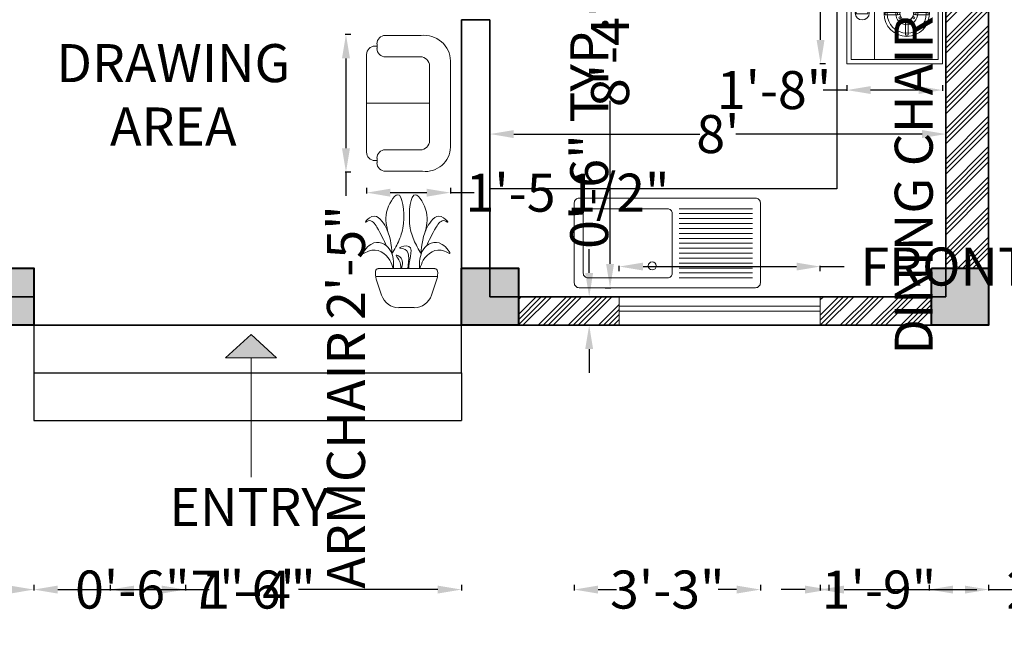
# Model space of a CAD drawing. Units: inches. Extents: x -52 to 493, y -432 to 100.
# Tile 2 of 5: x 163 to 370, y -432 to -300. Entities that reach past the tile are written whole.
import ezdxf

# ---------------------------------------------------------------- set-up
doc = ezdxf.new("R2010")
doc.units = ezdxf.units.IN
doc.header["$MEASUREMENT"] = 0
for name, color, linetype, lineweight in [('A-ANNO-DIMS', 2, 'Continuous', 18), ('A-ANNO-SYMB', 7, 'Continuous', 18), ('A-ANNO-TEXT', 7, 'Continuous', 25), ('A-AREA-IDEN', 7, 'Continuous', 25), ('A-COLS', 7, 'Continuous', 40), ('A-EQPM', 8, 'Continuous', 18), ('A-FLOR-CASE', 8, 'Continuous', 25), ('A-FLOR-FIXT', 9, 'Continuous', 18), ('A-FLOR-FIXT-PATT', 9, 'Continuous', 13), ('A-FLOR-STRS', 7, 'Continuous', 25), ('A-FURN', 8, 'Continuous', 18), ('A-GLAZ', 4, 'Continuous', 18), ('A-WALL', 7, 'Continuous', 35), ('A-WALL-PATT', 8, 'Continuous', 13)]:
    doc.layers.add(name, color=color, linetype=linetype, lineweight=lineweight)
doc.styles.get("Standard").update_dxf_attribs({"font": 'arial.ttf'})
doc.dimstyles.get("Standard").update_dxf_attribs({"dimtxt": 8, "dimasz": 5, "dimexe": 0.18, "dimexo": 0.0625, "dimgap": 0.09, "dimtad": 0, "dimdec": 0, "dimzin": 0, "dimdsep": 46, "dimlunit": 3, "dimtxsty": 'Standard', "dimcen": 0.09, "dimadec": 0, "dimazin": 0, "dimtfac": 1, "dimtdec": 0, "dimtofl": 0, "dimtmove": 0, "dimatfit": 3, "dimfxl": 1, "dimfxlon": 1, "dimtolj": 1, "dimtzin": 0, "dimarcsym": 0})

# ---------------------------------------------------------------- blocks, each defined once
blk = doc.blocks.new('A$C6D011943')
for p, q in [((1.448, 1.089), (0.332, 1.089)), ((1.364, 0.818), (0.398, 0.818)), ((0.881, 0.818), (0.881, 0)), ((0, 0.709), (0, 0.247)), ((0.278, 0.697), (0.278, 0.244)), ((1.485, 0.244), (1.485, 0.697)), ((1.762, 0.247), (1.762, 0.727)), ((0.109, 0.136), (0.169, 0.136)), ((0.139, 0.109), (0.139, 0.136)), ((1.593, 0.136), (1.654, 0.136)), ((1.648, 0.136), (1.623, 0.136)), ((1.623, 0.109), (1.623, 0.136)), ((1.515, 0), (0.247, 0))]:
    blk.add_line(p, q)
for centre, radius, start, end in [((0.339, 0.748), 0.342, 91.2564, 186.501), ((1.441, 0.766), 0.324, 353.159, 88.6697), ((0.398, 0.697), 0.121, 90, 180), ((1.364, 0.697), 0.121, 0, 90), ((0.109, 0.244), 0.109, 180, 270), ((0.169, 0.244), 0.109, 270, 0), ((1.593, 0.244), 0.109, 180, 270), ((1.654, 0.244), 0.109, 270, 0), ((0.247, 0.109), 0.109, 180, 270), ((1.515, 0.109), 0.109, 270, 0)]:
    blk.add_arc(centre, radius, start, end)
blk = doc.blocks.new('A$C06E242FC')
for p, q in [((0, 455.6), (0.5, 456.1)), ((0, 455.6), (0, 0.5)), ((838.9, 456.1), (0.5, 456.1)), ((20, 435.6), (20.5, 436.1)), ((20, 435.6), (20, 20.5)), ((818.9, 436.1), (20.5, 436.1)), ((819.4, 435.6), (818.9, 436.1)), ((819.4, 20.5), (819.4, 435.6)), ((838.9, 456.1), (839.4, 455.6)), ((839.4, 0.5), (839.4, 455.6)), ((237.3, 411.5), (237.3, 356.2)), ((248.9, 411.5), (237.3, 411.5)), ((248.9, 356.2), (248.9, 411.5)), ((599.3, 411.5), (610.9, 411.5)), ((599.3, 411.5), (599.3, 356.2)), ((610.9, 356.2), (610.9, 411.5)), ((237.3, 356.2), (248.9, 356.2)), ((599.3, 356.2), (610.9, 356.2)), ((20, 324.4), (819.4, 324.4)), ((232.7, 272.7), (232.7, 214)), ((244.9, 272.7), (232.7, 272.7)), ((244.9, 214), (244.9, 272.7)), ((588.1, 272.7), (588.1, 214)), ((600.3, 272.7), (588.1, 272.7)), ((600.3, 214), (600.3, 272.7)), ((232.7, 214), (244.9, 214)), ((588.1, 214), (600.3, 214)), ((136.3, 176), (136.3, 163.8)), ((194.9, 176), (136.3, 176)), ((136.3, 163.8), (194.9, 163.8)), ((194.9, 163.8), (194.9, 176)), ((282.9, 176.3), (282.9, 164.1)), ((341.6, 176.3), (282.9, 176.3)), ((282.9, 164.1), (341.6, 164.1)), ((341.6, 164.1), (341.6, 176.3)), ((550.3, 176), (491.7, 176)), ((491.7, 176), (491.7, 163.8)), ((491.7, 163.8), (550.3, 163.8)), ((550.3, 163.8), (550.3, 176)), ((638.3, 176.3), (638.3, 164.1)), ((697, 176.3), (638.3, 176.3)), ((638.3, 164.1), (697, 164.1)), ((697, 164.1), (697, 176.3)), ((245.2, 126.1), (233, 126.1)), ((233, 126.1), (233, 67.4)), ((245.2, 67.4), (245.2, 126.1)), ((600.6, 126.1), (588.3, 126.1)), ((588.3, 126.1), (588.3, 67.4)), ((600.6, 67.4), (600.6, 126.1)), ((233, 67.4), (245.2, 67.4)), ((588.3, 67.4), (600.6, 67.4)), ((0, 0.5), (0.5, 0)), ((20, 20.5), (20.5, 20)), ((20.5, 20), (818.9, 20)), ((818.9, 20), (819.4, 20.5)), ((838.9, 0), (839.4, 0.5)), ((0.5, 0), (838.9, 0))]:
    blk.add_line(p, q)
for centre, radius in [((242, 382.9), 33.3), ((604.1, 382.9), 33.3), ((238.9, 170.1), 108.3), ((238.9, 170.1), 93.3), ((594.3, 170.1), 108.3), ((594.3, 170.1), 93.3), ((238.9, 170.1), 52.6), ((205.3, 189.5), 4.84), ((238.9, 170.1), 32.6), ((219.5, 203.7), 4.84), ((238.9, 208.9), 4.84), ((258.4, 203.7), 4.84), ((272.6, 189.5), 4.84), ((594.3, 170.1), 52.6), ((560.7, 189.5), 4.84), ((594.3, 170.1), 32.6), ((574.9, 203.7), 4.84), ((594.3, 208.9), 4.84), ((613.7, 203.7), 4.84), ((628, 189.5), 4.84), ((200.1, 170.1), 4.84), ((205.3, 150.6), 4.84), ((219.5, 136.4), 4.84), ((258.4, 136.4), 4.84), ((272.6, 150.6), 4.84), ((277.8, 170.1), 4.84), ((555.5, 170.1), 4.84), ((560.7, 150.6), 4.84), ((574.9, 136.4), 4.84), ((613.7, 136.4), 4.84), ((628, 150.6), 4.84), ((633.2, 170.1), 4.84), ((238.9, 131.2), 4.84), ((594.3, 131.2), 4.84)]:
    blk.add_circle(centre, radius)
blk = doc.blocks.new('*D19')
at = {"layer": 'A-ANNO-DIMS', "color": 0, "lineweight": -2, "transparency": 16777216}
for p, q in [((285.94, -256.62), (287.12, -256.62)), ((286.94, -261.62), (286.94, -295.94)), ((286.94, -351.72), (286.94, -317.4)), ((285.94, -356.72), (287.12, -356.72))]:
    blk.add_line(p, q, dxfattribs=at)
at = {"layer": 'A-ANNO-DIMS', "color": 0, "transparency": 16777216}
for points in [[(286.11, -261.62), (287.78, -261.62), (286.94, -256.62)], [(286.11, -351.72), (287.78, -351.72), (286.94, -356.72)]]:
    blk.add_solid(points, dxfattribs=at)
at = {"layer": 'Defpoints', "color": 0, "transparency": 16777216}
for p in [(283.02, -256.62), (280.41, -356.72), (286.94, -356.72)]:
    blk.add_point(p, dxfattribs=at)
at = {"layer": 'A-ANNO-DIMS', "color": 0, "transparency": 16777216, "insert": (286.94, -306.67), "char_height": 8, "attachment_point": 5, "rotation": 90}
blk.add_mtext('\\A1;8\'-4"', dxfattribs=at)
blk = doc.blocks.new('*D20')
at = {"layer": 'A-ANNO-DIMS', "color": 0, "lineweight": -2, "transparency": 16777216}
for p, q in [((261.65, -323.39), (261.65, -324.57)), ((266.65, -324.39), (305.87, -324.39)), ((352.65, -324.39), (313.42, -324.39)), ((357.65, -323.39), (357.65, -324.57))]:
    blk.add_line(p, q, dxfattribs=at)
at = {"layer": 'A-ANNO-DIMS', "color": 0, "transparency": 16777216}
for points in [[(266.65, -323.56), (266.65, -325.23), (261.65, -324.39)], [(352.65, -323.56), (352.65, -325.23), (357.65, -324.39)]]:
    blk.add_solid(points, dxfattribs=at)
at = {"layer": 'Defpoints', "color": 0, "transparency": 16777216}
for p in [(261.65, -318.52), (357.65, -318.52), (357.65, -324.39)]:
    blk.add_point(p, dxfattribs=at)
at = {"layer": 'A-ANNO-DIMS', "color": 0, "transparency": 16777216, "insert": (309.65, -324.39), "char_height": 8, "attachment_point": 5}
blk.add_mtext("\\A1;8'", dxfattribs=at)
blk = doc.blocks.new('COL-12X12')
h = blk.add_hatch(color=256)
h.dxf.hatch_style = 1
h.paths.add_polyline_path([(12, 12), (0, 12), (0, 0), (12, 0)])
blk.add_lwpolyline([(0, 12), (12, 12), (12, 0), (0, 0)], close=True)
blk = doc.blocks.new('WIN-FRONT-42')
for p, q in [((0, 6), (0, 0)), ((42.31, 6), (42.31, 0)), ((42.31, 4), (0, 4)), ((42.31, 3), (0, 3))]:
    blk.add_line(p, q)
blk = doc.blocks.new('*D36')
at = {"layer": 'A-ANNO-DIMS', "color": 0, "lineweight": -2, "transparency": 16777216}
for p, q in [((288.89, -353.27), (288.89, -352.09)), ((293.89, -352.27), (326.2, -352.27)), ((331.2, -353.27), (331.2, -352.09)), ((331.2, -352.27), (336.2, -352.27))]:
    blk.add_line(p, q, dxfattribs=at)
at = {"layer": 'A-ANNO-DIMS', "color": 0, "transparency": 16777216}
for points in [[(293.89, -351.44), (293.89, -353.1), (288.89, -352.27)], [(326.2, -351.44), (326.2, -353.1), (331.2, -352.27)]]:
    blk.add_solid(points, dxfattribs=at)
at = {"layer": 'Defpoints', "color": 0, "transparency": 16777216}
for p in [(331.2, -352.27), (288.89, -358.62), (331.2, -358.62)]:
    blk.add_point(p, dxfattribs=at)
at = {"layer": 'A-ANNO-DIMS', "color": 0, "transparency": 16777216, "insert": (416.63, -352.27), "char_height": 8, "attachment_point": 5}
blk.add_mtext('\\A1;FRONT WINDOW 3\'-6 1/2" TYP.', dxfattribs=at)
blk = doc.blocks.new('*D37')
at = {"layer": 'A-ANNO-DIMS', "color": 0, "lineweight": -2, "transparency": 16777216}
for p, q in [((282.55, -353.62), (282.55, -348.62)), ((283.55, -358.62), (282.37, -358.62)), ((283.55, -364.62), (282.37, -364.62)), ((282.55, -369.62), (282.55, -374.62))]:
    blk.add_line(p, q, dxfattribs=at)
at = {"layer": 'A-ANNO-DIMS', "color": 0, "transparency": 16777216}
for points in [[(281.71, -353.62), (283.38, -353.62), (282.55, -358.62)], [(281.71, -369.62), (283.38, -369.62), (282.55, -364.62)]]:
    blk.add_solid(points, dxfattribs=at)
at = {"layer": 'Defpoints', "color": 0, "transparency": 16777216}
for p in [(282.55, -358.62), (288.89, -358.62), (288.89, -364.62)]:
    blk.add_point(p, dxfattribs=at)
at = {"layer": 'A-ANNO-DIMS', "color": 0, "transparency": 16777216, "insert": (282.55, -324.14), "char_height": 8, "attachment_point": 5, "rotation": 90}
blk.add_mtext('\\A1;0\'-6" TYP.', dxfattribs=at)
blk = doc.blocks.new('*D44')
at = {"layer": 'A-ANNO-DIMS', "color": 0, "lineweight": -2, "transparency": 16777216}
for p, q in [((349.88, -208.05), (351.06, -208.05)), ((350.88, -213.05), (350.88, -216.46)), ((349.88, -221.46), (351.06, -221.46)), ((350.88, -221.46), (350.88, -226.46))]:
    blk.add_line(p, q, dxfattribs=at)
at = {"layer": 'A-ANNO-DIMS', "color": 0, "transparency": 16777216}
for points in [[(350.04, -213.05), (351.71, -213.05), (350.88, -208.05)], [(350.04, -216.46), (351.71, -216.46), (350.88, -221.46)]]:
    blk.add_solid(points, dxfattribs=at)
at = {"layer": 'Defpoints', "color": 0, "transparency": 16777216}
for p in [(348.87, -208.05), (348.87, -221.46), (350.88, -221.46)]:
    blk.add_point(p, dxfattribs=at)
at = {"layer": 'A-ANNO-DIMS', "color": 0, "transparency": 16777216, "insert": (350.88, -300.1), "char_height": 8, "attachment_point": 5, "rotation": 90}
blk.add_mtext('\\A1;DINING CHAIR 1\'-1 1/2" TYP.', dxfattribs=at)
blk = doc.blocks.new('*D52')
at = {"layer": 'A-ANNO-DIMS', "color": 0, "lineweight": -2, "transparency": 16777216}
for p, q in [((232.34, -303.47), (231.16, -303.47)), ((231.34, -308.47), (231.34, -327.39)), ((232.34, -332.39), (231.16, -332.39)), ((231.34, -332.39), (231.34, -337.39))]:
    blk.add_line(p, q, dxfattribs=at)
at = {"layer": 'A-ANNO-DIMS', "color": 0, "transparency": 16777216}
for points in [[(230.51, -308.47), (232.18, -308.47), (231.34, -303.47)], [(230.51, -327.39), (232.18, -327.39), (231.34, -332.39)]]:
    blk.add_solid(points, dxfattribs=at)
at = {"layer": 'Defpoints', "color": 0, "transparency": 16777216}
for p in [(235.68, -303.47), (231.34, -332.39), (235.68, -332.39)]:
    blk.add_point(p, dxfattribs=at)
at = {"layer": 'A-ANNO-DIMS', "color": 0, "transparency": 16777216, "insert": (231.34, -379.7), "char_height": 8, "attachment_point": 5, "rotation": 90}
blk.add_mtext('\\A1;ARMCHAIR 2\'-5"', dxfattribs=at)
blk = doc.blocks.new('*D53')
at = {"layer": 'A-ANNO-DIMS', "color": 0, "lineweight": -2, "transparency": 16777216}
for p, q in [((235.68, -335.72), (235.68, -336.9)), ((253.34, -335.72), (253.34, -336.9)), ((240.68, -336.72), (248.34, -336.72)), ((253.34, -336.72), (258.34, -336.72))]:
    blk.add_line(p, q, dxfattribs=at)
at = {"layer": 'A-ANNO-DIMS', "color": 0, "transparency": 16777216}
for points in [[(240.68, -335.89), (240.68, -337.56), (235.68, -336.72)], [(248.34, -335.89), (248.34, -337.56), (253.34, -336.72)]]:
    blk.add_solid(points, dxfattribs=at)
at = {"layer": 'Defpoints', "color": 0, "transparency": 16777216}
for p in [(235.68, -332.39), (253.34, -332.39), (253.34, -336.72)]:
    blk.add_point(p, dxfattribs=at)
at = {"layer": 'A-ANNO-DIMS', "color": 0, "transparency": 16777216, "insert": (278, -336.72), "char_height": 8, "attachment_point": 5}
blk.add_mtext('\\A1;1\'-5 1/2"', dxfattribs=at)
blk = doc.blocks.new('*D54')
at = {"layer": 'A-ANNO-DIMS', "color": 0, "lineweight": -2, "transparency": 16777216}
for p, q in [((331.27, -272.61), (331.27, -267.61)), ((332.27, -272.61), (331.09, -272.61)), ((331.27, -304.59), (331.27, -277.61)), ((332.27, -309.59), (331.09, -309.59))]:
    blk.add_line(p, q, dxfattribs=at)
at = {"layer": 'A-ANNO-DIMS', "color": 0, "transparency": 16777216}
for points in [[(330.43, -277.61), (332.1, -277.61), (331.27, -272.61)], [(330.43, -304.59), (332.1, -304.59), (331.27, -309.59)]]:
    blk.add_solid(points, dxfattribs=at)
at = {"layer": 'Defpoints', "color": 0, "transparency": 16777216}
for p in [(331.27, -272.61), (336.81, -272.61), (336.81, -309.59)]:
    blk.add_point(p, dxfattribs=at)
at = {"layer": 'A-ANNO-DIMS', "color": 0, "transparency": 16777216, "insert": (331.27, -227.44), "char_height": 8, "attachment_point": 5, "rotation": 90}
blk.add_mtext('\\A1;COOKTOP 3\'-1"', dxfattribs=at)
blk = doc.blocks.new('*D55')
at = {"layer": 'A-ANNO-DIMS', "color": 0, "lineweight": -2, "transparency": 16777216}
for p, q in [((336.81, -314.14), (336.81, -315.32)), ((356.91, -314.14), (356.91, -315.32)), ((336.81, -315.14), (331.81, -315.14)), ((351.91, -315.14), (341.81, -315.14))]:
    blk.add_line(p, q, dxfattribs=at)
at = {"layer": 'A-ANNO-DIMS', "color": 0, "transparency": 16777216}
for points in [[(341.81, -314.31), (341.81, -315.97), (336.81, -315.14)], [(351.91, -314.31), (351.91, -315.97), (356.91, -315.14)]]:
    blk.add_solid(points, dxfattribs=at)
at = {"layer": 'Defpoints', "color": 0, "transparency": 16777216}
for p in [(336.81, -309.59), (356.91, -309.59), (336.81, -315.14)]:
    blk.add_point(p, dxfattribs=at)
at = {"layer": 'A-ANNO-DIMS', "color": 0, "transparency": 16777216, "insert": (321.47, -315.14), "char_height": 8, "attachment_point": 5}
blk.add_mtext('\\A1;1\'-8"', dxfattribs=at)
blk = doc.blocks.new('*D64')
at = {"layer": 'A-ANNO-DIMS', "color": 0, "lineweight": -2, "transparency": 16777216}
for p, q in [((101.4, -419.22), (101.4, -420.4)), ((106.4, -420.22), (113.48, -420.22)), ((160.65, -420.22), (153.57, -420.22)), ((165.65, -419.22), (165.65, -420.4))]:
    blk.add_line(p, q, dxfattribs=at)
at = {"layer": 'A-ANNO-DIMS', "color": 0, "transparency": 16777216}
for points in [[(106.4, -419.39), (106.4, -421.06), (101.4, -420.22)], [(160.65, -419.39), (160.65, -421.06), (165.65, -420.22)]]:
    blk.add_solid(points, dxfattribs=at)
at = {"layer": 'Defpoints', "color": 0, "transparency": 16777216}
for p in [(101.4, -364.62), (165.65, -364.62), (165.65, -420.22)]:
    blk.add_point(p, dxfattribs=at)
at = {"layer": 'A-ANNO-DIMS', "color": 0, "transparency": 16777216, "insert": (133.52, -420.22), "char_height": 8, "attachment_point": 5}
blk.add_mtext('\\A1;5\'-4 1/2"', dxfattribs=at)
blk = doc.blocks.new('*D65')
at = {"layer": 'A-ANNO-DIMS', "color": 0, "lineweight": -2, "transparency": 16777216}
for p, q in [((331.2, -419.22), (331.2, -420.4)), ((336.2, -420.22), (361.65, -420.22)), ((366.65, -419.22), (366.65, -420.4)), ((366.65, -420.22), (371.65, -420.22))]:
    blk.add_line(p, q, dxfattribs=at)
at = {"layer": 'A-ANNO-DIMS', "color": 0, "transparency": 16777216}
for points in [[(336.2, -419.39), (336.2, -421.06), (331.2, -420.22)], [(361.65, -419.39), (361.65, -421.06), (366.65, -420.22)]]:
    blk.add_solid(points, dxfattribs=at)
at = {"layer": 'Defpoints', "color": 0, "transparency": 16777216}
for p in [(331.2, -364.62), (366.65, -364.62), (366.65, -420.22)]:
    blk.add_point(p, dxfattribs=at)
at = {"layer": 'A-ANNO-DIMS', "color": 0, "transparency": 16777216, "insert": (394.87, -420.22), "char_height": 8, "attachment_point": 5}
blk.add_mtext('\\A1;2\'-11 1/2"', dxfattribs=at)
blk = doc.blocks.new('*D66')
at = {"layer": 'A-ANNO-DIMS', "color": 0, "lineweight": -2, "transparency": 16777216}
for p, q in [((389.3, -364.62), (390.48, -364.62)), ((390.3, -369.62), (390.3, -379.62)), ((389.3, -384.62), (390.48, -384.62)), ((390.3, -384.62), (390.3, -389.62))]:
    blk.add_line(p, q, dxfattribs=at)
at = {"layer": 'A-ANNO-DIMS', "color": 0, "transparency": 16777216}
for points in [[(389.46, -369.62), (391.13, -369.62), (390.3, -364.62)], [(389.46, -379.62), (391.13, -379.62), (390.3, -384.62)]]:
    blk.add_solid(points, dxfattribs=at)
at = {"layer": 'Defpoints', "color": 0, "transparency": 16777216}
for p in [(255.65, -364.62), (255.65, -384.62), (390.3, -384.62)]:
    blk.add_point(p, dxfattribs=at)
at = {"layer": 'A-ANNO-DIMS', "color": 0, "transparency": 16777216, "insert": (390.3, -399.96), "char_height": 8, "attachment_point": 5, "rotation": 90}
blk.add_mtext('\\A1;1\'-8"', dxfattribs=at)
blk = doc.blocks.new('*D67')
at = {"layer": 'A-ANNO-DIMS', "color": 0, "lineweight": -2, "transparency": 16777216}
for p, q in [((165.65, -419.22), (165.65, -420.4)), ((170.65, -420.22), (199.96, -420.22)), ((250.65, -420.22), (221.34, -420.22)), ((255.65, -419.22), (255.65, -420.4))]:
    blk.add_line(p, q, dxfattribs=at)
at = {"layer": 'A-ANNO-DIMS', "color": 0, "transparency": 16777216}
for points in [[(170.65, -419.39), (170.65, -421.06), (165.65, -420.22)], [(250.65, -419.39), (250.65, -421.06), (255.65, -420.22)]]:
    blk.add_solid(points, dxfattribs=at)
at = {"layer": 'Defpoints', "color": 0, "transparency": 16777216}
for p in [(165.65, -384.62), (255.65, -384.62), (255.65, -420.22)]:
    blk.add_point(p, dxfattribs=at)
at = {"layer": 'A-ANNO-DIMS', "color": 0, "transparency": 16777216, "insert": (210.65, -420.22), "char_height": 8, "attachment_point": 5}
blk.add_mtext('\\A1;7\'-6"', dxfattribs=at)
blk = doc.blocks.new('*D74')
at = {"layer": 'A-ANNO-DIMS', "color": 0, "lineweight": -2, "transparency": 16777216}
for p, q in [((334.72, 87.29), (334.72, 88.47)), ((339.72, 88.29), (352.65, 88.29)), ((357.65, 87.29), (357.65, 88.47)), ((357.65, 88.29), (362.65, 88.29))]:
    blk.add_line(p, q, dxfattribs=at)
at = {"layer": 'A-ANNO-DIMS', "color": 0, "transparency": 16777216}
for points in [[(339.72, 89.13), (339.72, 87.46), (334.72, 88.29)], [(352.65, 89.13), (352.65, 87.46), (357.65, 88.29)]]:
    blk.add_solid(points, dxfattribs=at)
at = {"layer": 'Defpoints', "color": 0, "transparency": 16777216}
for p in [(357.65, 88.29), (334.72, -335.93), (357.65, -358.62)]:
    blk.add_point(p, dxfattribs=at)
at = {"layer": 'A-ANNO-DIMS', "color": 0, "transparency": 16777216, "insert": (376.1, 88.29), "char_height": 8, "attachment_point": 5}
blk.add_mtext('\\A1;1\'-11"', dxfattribs=at)
blk = doc.blocks.new('*D75')
at = {"layer": 'A-ANNO-DIMS', "color": 0, "lineweight": -2, "transparency": 16777216}
for p, q in [((389.3, -335.93), (390.48, -335.93)), ((390.3, -340.93), (390.3, -353.62)), ((389.3, -358.62), (390.48, -358.62)), ((390.3, -358.62), (390.3, -363.62))]:
    blk.add_line(p, q, dxfattribs=at)
at = {"layer": 'A-ANNO-DIMS', "color": 0, "transparency": 16777216}
for points in [[(389.46, -340.93), (391.13, -340.93), (390.3, -335.93)], [(389.46, -353.62), (391.13, -353.62), (390.3, -358.62)]]:
    blk.add_solid(points, dxfattribs=at)
at = {"layer": 'Defpoints', "color": 0, "transparency": 16777216}
for p in [(334.72, -335.93), (331.2, -358.62), (390.3, -358.62)]:
    blk.add_point(p, dxfattribs=at)
at = {"layer": 'A-ANNO-DIMS', "color": 0, "transparency": 16777216, "insert": (390.3, -386.39), "char_height": 8, "attachment_point": 5, "rotation": 90}
blk.add_mtext('\\A1;1\'-10 1/2"', dxfattribs=at)
blk = doc.blocks.new('*D76')
at = {"layer": 'A-ANNO-DIMS', "color": 0, "lineweight": -2, "transparency": 16777216}
for p, q in [((327.99, -420.22), (322.99, -420.22)), ((332.99, -419.22), (332.99, -420.4)), ((354.16, -419.22), (354.16, -420.4)), ((359.16, -420.22), (364.16, -420.22))]:
    blk.add_line(p, q, dxfattribs=at)
at = {"layer": 'A-ANNO-DIMS', "color": 0, "transparency": 16777216}
for points in [[(327.99, -419.39), (327.99, -421.06), (332.99, -420.22)], [(359.16, -419.39), (359.16, -421.06), (354.16, -420.22)]]:
    blk.add_solid(points, dxfattribs=at)
at = {"layer": 'Defpoints', "color": 0, "transparency": 16777216}
for p in [(332.99, -208.05), (354.16, -208.05), (354.16, -420.22)]:
    blk.add_point(p, dxfattribs=at)
at = {"layer": 'A-ANNO-DIMS', "color": 0, "transparency": 16777216, "insert": (343.57, -420.22), "char_height": 8, "attachment_point": 5}
blk.add_mtext('\\A1;1\'-9"', dxfattribs=at)
blk = doc.blocks.new('*D79')
at = {"layer": 'A-ANNO-DIMS', "color": 0, "lineweight": -2, "transparency": 16777216}
for p, q in [((181.73, -419.22), (181.73, -420.4)), ((186.73, -420.22), (192.57, -420.22)), ((197.57, -419.22), (197.57, -420.4)), ((197.57, -420.22), (202.57, -420.22))]:
    blk.add_line(p, q, dxfattribs=at)
at = {"layer": 'A-ANNO-DIMS', "color": 0, "transparency": 16777216}
for points in [[(186.73, -419.39), (186.73, -421.06), (181.73, -420.22)], [(192.57, -419.39), (192.57, -421.06), (197.57, -420.22)]]:
    blk.add_solid(points, dxfattribs=at)
at = {"layer": 'Defpoints', "color": 0, "transparency": 16777216}
for p in [(181.73, 19.38), (197.57, 19.38), (197.57, -420.22)]:
    blk.add_point(p, dxfattribs=at)
at = {"layer": 'A-ANNO-DIMS', "color": 0, "transparency": 16777216, "insert": (212.91, -420.22), "char_height": 8, "attachment_point": 5}
blk.add_mtext('\\A1;1\'-4"', dxfattribs=at)
blk = doc.blocks.new('*D81')
at = {"layer": 'A-ANNO-DIMS', "color": 0, "lineweight": -2, "transparency": 16777216}
for p, q in [((154.65, -420.22), (149.65, -420.22)), ((159.65, -419.22), (159.65, -420.4)), ((165.65, -419.22), (165.65, -420.4)), ((170.65, -420.22), (175.65, -420.22))]:
    blk.add_line(p, q, dxfattribs=at)
at = {"layer": 'A-ANNO-DIMS', "color": 0, "transparency": 16777216}
for points in [[(154.65, -419.39), (154.65, -421.06), (159.65, -420.22)], [(170.65, -419.39), (170.65, -421.06), (165.65, -420.22)]]:
    blk.add_solid(points, dxfattribs=at)
at = {"layer": 'Defpoints', "color": 0, "transparency": 16777216}
for p in [(159.65, -79.87), (165.65, -79.87), (165.65, -420.22)]:
    blk.add_point(p, dxfattribs=at)
at = {"layer": 'A-ANNO-DIMS', "color": 0, "transparency": 16777216, "insert": (186.37, -420.22), "char_height": 8, "attachment_point": 5}
blk.add_mtext('\\A1;0\'-6"', dxfattribs=at)
blk = doc.blocks.new('*D82')
at = {"layer": 'A-ANNO-DIMS', "color": 0, "lineweight": -2, "transparency": 16777216}
for p, q in [((279.41, -419.22), (279.41, -420.4)), ((284.41, -420.22), (288.28, -420.22)), ((313.59, -420.22), (309.72, -420.22)), ((318.59, -419.22), (318.59, -420.4))]:
    blk.add_line(p, q, dxfattribs=at)
at = {"layer": 'A-ANNO-DIMS', "color": 0, "transparency": 16777216}
for points in [[(284.41, -419.39), (284.41, -421.06), (279.41, -420.22)], [(313.59, -419.39), (313.59, -421.06), (318.59, -420.22)]]:
    blk.add_solid(points, dxfattribs=at)
at = {"layer": 'Defpoints', "color": 0, "transparency": 16777216}
for p in [(279.41, -338.87), (318.59, -338.87), (318.59, -420.22)]:
    blk.add_point(p, dxfattribs=at)
at = {"layer": 'A-ANNO-DIMS', "color": 0, "transparency": 16777216, "insert": (299, -420.22), "char_height": 8, "attachment_point": 5}
blk.add_mtext('\\A1;3\'-3"', dxfattribs=at)
blk = doc.blocks.new('*D83')
at = {"layer": 'A-ANNO-DIMS', "color": 0, "lineweight": -2, "transparency": 16777216}
for p, q in [((389.3, -337.87), (390.48, -337.87)), ((390.3, -342.87), (390.3, -351.72)), ((389.3, -356.72), (390.48, -356.72)), ((390.3, -356.72), (390.3, -361.72))]:
    blk.add_line(p, q, dxfattribs=at)
at = {"layer": 'A-ANNO-DIMS', "color": 0, "transparency": 16777216}
for points in [[(389.46, -342.87), (391.13, -342.87), (390.3, -337.87)], [(389.46, -351.72), (391.13, -351.72), (390.3, -356.72)]]:
    blk.add_solid(points, dxfattribs=at)
at = {"layer": 'Defpoints', "color": 0, "transparency": 16777216}
for p in [(280.41, -337.87), (280.41, -356.72), (390.3, -356.72)]:
    blk.add_point(p, dxfattribs=at)
at = {"layer": 'A-ANNO-DIMS', "color": 0, "transparency": 16777216, "insert": (390.3, -372.07), "char_height": 8, "attachment_point": 5, "rotation": 90}
blk.add_mtext('\\A1;1\'-7"', dxfattribs=at)
blk = doc.blocks.new('*D84')
at = {"layer": 'A-ANNO-DIMS', "color": 0, "lineweight": -2, "transparency": 16777216}
for p, q in [((349.33, -283.41), (349.51, -283.41)), ((349.42, -283.5), (349.42, -283.32)), ((364.19, -283.41), (359.19, -283.41))]:
    blk.add_line(p, q, dxfattribs=at)
at = {"layer": 'A-ANNO-DIMS', "color": 0, "transparency": 16777216}
blk.add_solid([(359.19, -282.58), (359.19, -284.25), (354.19, -283.41)], dxfattribs=at)
at = {"layer": 'Defpoints', "color": 0, "transparency": 16777216}
for p in [(344.65, -283.41), (354.19, -283.41)]:
    blk.add_point(p, dxfattribs=at)
at = {"layer": 'A-ANNO-DIMS', "color": 0, "transparency": 16777216, "insert": (397.03, -283.42), "char_height": 8, "attachment_point": 5, "rotation": 359.9944}
blk.add_mtext('\\A1;2X ∅0\'-9 1/2"', dxfattribs=at)

msp = doc.modelspace()

# ---------------------------------------------------------------- hatches: boundary and pattern name
at = {"layer": 'A-ANNO-SYMB'}
h = msp.add_hatch(color=256, dxfattribs=at)
h.dxf.hatch_style = 1
h.paths.add_polyline_path([(211.37, -366.55), (206.01, -371.48), (211.37, -371.48), (216.72, -371.48)])
at = {"layer": 'A-FLOR-FIXT-PATT'}
h = msp.add_hatch(dxfattribs=at)
h.set_pattern_fill('ANSI31', color=256, scale=8.3204, angle=-45, style=0)
h.paths.add_polyline_path([(301.49, -355.13), (316.93, -355.13), (316.93, -339.62), (301.49, -339.62)])
at = {"layer": 'A-WALL-PATT'}
h = msp.add_hatch(dxfattribs=at)
h.set_pattern_fill('ANSI34', color=256, scale=6)
h.paths.add_polyline_path([(366.65, -213.25), (357.65, -213.25), (357.65, -247.89), (366.65, -247.89)])
h.paths.add_polyline_path([(354.65, -250.62), (267.65, -250.62), (267.65, -256.62), (354.65, -256.62)])
h.paths.add_polyline_path([(366.65, -259.89), (357.65, -259.89), (357.65, -352.62), (366.65, -352.62)])
h.paths.add_polyline_path([(354.65, -358.62), (331.2, -358.62), (331.2, -364.62), (354.65, -364.62)])
h.paths.add_polyline_path([(288.89, -358.62), (267.65, -358.62), (267.65, -364.62), (288.89, -364.62)])
h.paths.add_polyline_path([(153.65, -358.62), (101.4, -358.62), (101.4, -364.62), (153.65, -364.62)])
h.paths.add_polyline_path([(59.09, -358.62), (18.65, -358.62), (18.65, -364.62), (59.09, -364.62)])
h.paths.add_polyline_path([(15.65, -259.14), (6.65, -259.14), (6.65, -352.62), (15.65, -352.62)])
h.paths.add_polyline_path([(153.65, -250.62), (18.65, -250.62), (18.65, -256.62), (153.65, -256.62)])
h.paths.add_polyline_path([(15.65, -213.25), (6.65, -213.25), (6.65, -247.14), (15.65, -247.14)])
h.paths.add_polyline_path([(15.65, -121.57), (6.65, -121.57), (6.65, -155.46), (15.65, -155.46), (15.65, -143.44)])

# ---------------------------------------------------------------- linework, layer by layer
at = {"layer": 'A-ANNO-SYMB'}
for p, q in [((206.01, -371.48), (211.37, -366.55)), ((216.72, -371.48), (211.37, -366.55)), ((211.37, -371.48), (206.01, -371.48)), ((211.37, -396.57), (211.37, -371.48)), ((211.37, -371.48), (216.72, -371.48))]:
    msp.add_line(p, q, dxfattribs=at)
at = {"layer": 'A-FLOR-CASE'}
for p, q in [((334.72, -256.62), (334.72, -335.93)), ((334.72, -335.93), (261.65, -335.93))]:
    msp.add_line(p, q, dxfattribs=at)
at = {"layer": 'A-FLOR-FIXT'}
for points in [[(280.41, -337.87), (317.59, -337.87, -0.414214), (318.59, -338.87), (318.59, -355.72, -0.414214), (317.59, -356.72), (280.41, -356.72, -0.414214), (279.41, -355.72), (279.41, -338.87, -0.414214)], [(282.31, -340.09), (299.03, -340.09, -0.414214), (300.03, -341.09), (300.03, -353.67, -0.414214), (299.03, -354.67), (282.31, -354.67, -0.414214), (281.31, -353.67), (281.31, -341.09, -0.414214)]]:
    msp.add_lwpolyline(points, format="xyb", close=True, dxfattribs=at)
msp.add_circle((295.82, -352.12), 0.848, dxfattribs=at)
at = {"layer": 'A-FLOR-STRS'}
for p, q in [((165.65, -364.62), (165.65, -374.62)), ((255.65, -374.62), (255.65, -364.62)), ((165.65, -374.62), (255.65, -374.62)), ((165.65, -374.62), (165.65, -384.62)), ((255.65, -374.62), (255.65, -384.62)), ((165.65, -384.62), (255.65, -384.62))]:
    msp.add_line(p, q, dxfattribs=at)
at = {"layer": 'A-FURN'}
for p, q in [((237.58, -354.35), (250.6, -354.35)), ((238.11, -352.71), (250.07, -352.71)), ((237.73, -354.94), (238.85, -358.3)), ((250.46, -354.94), (249.34, -358.3)), ((242.48, -360.91), (245.71, -360.91))]:
    msp.add_line(p, q, dxfattribs=at)
for centre, radius, start, end in [((241.36, -353.73), 3.83, 171.7201, 198.4349), ((238.11, -353.26), 0.547, 90, 171.7201), ((250.07, -353.26), 0.547, 8.2799, 90), ((246.83, -353.73), 3.83, 341.5651, 8.2799), ((242.48, -357.09), 3.83, 198.4349, 270), ((245.71, -357.09), 3.83, 270, 341.5651)]:
    msp.add_arc(centre, radius, start, end, dxfattribs=at)
for points, knots in [([(240.25, -345.15), (239.88, -343.81), (239.16, -341.14), (243.04, -334.45), (243.88, -342.89), (242.7, -346.56), (241.58, -348.64), (241.03, -349.64)], [0, 0, 0, 0, 4.327003, 8.661535, 14.827696, 18.413446, 21.747479, 21.747479, 21.747479, 21.747479]), ([(247.94, -345.15), (248.3, -343.81), (249.03, -341.14), (245.15, -334.45), (244.31, -342.89), (245.48, -346.56), (246.61, -348.64), (247.15, -349.64)], [0, 0, 0, 0, 4.327003, 8.661535, 14.827696, 18.413446, 21.747479, 21.747479, 21.747479, 21.747479]), ([(239.89, -347.93), (239.32, -346.72), (238.45, -344.89), (236.69, -342.13), (235, -343.28), (237.3, -340.57), (240.68, -344.64), (240.9, -347.69), (241.03, -349.64)], [0, 0, 0, 0, 4.426329, 6.700861, 7.332185, 8.618819, 12.199634, 18.436118, 18.436118, 18.436118, 18.436118]), ([(248.3, -347.93), (248.87, -346.72), (249.73, -344.89), (251.5, -342.13), (253.19, -343.28), (250.88, -340.57), (247.5, -344.64), (247.29, -347.69), (247.15, -349.64)], [0, 0, 0, 0, 4.426329, 6.700861, 7.332185, 8.618819, 12.199634, 18.436118, 18.436118, 18.436118, 18.436118]), ([(241.27, -352.71), (241.08, -352.1), (240.43, -349.97), (237.54, -347.98), (234.22, -350.15), (237.25, -346.01), (241.36, -348.44), (241.38, -351.37), (241.38, -352.73), (241.38, -352.74)], [0, 0, 0, 0, 1.920011, 6.760126, 7.950721, 10.437859, 14.588056, 18.647049, 18.678234, 18.678234, 18.678234, 18.678234]), ([(244.34, -352.71), (244.64, -350.74), (244.98, -348.52), (242.08, -348.39), (246.29, -346.96), (244.51, -350.99), (244.57, -352.54), (244.57, -352.71)], [0, 0, 0, 0, 4.388056, 4.951946, 6.423915, 10.705061, 11.24684, 11.24684, 11.24684, 11.24684]), ([(246.92, -352.71), (247.1, -352.1), (247.76, -349.97), (250.65, -347.98), (253.96, -350.15), (250.94, -346.01), (246.83, -348.44), (246.81, -351.37), (246.81, -352.73), (246.81, -352.74)], [0, 0, 0, 0, 1.920011, 6.760126, 7.950721, 10.437859, 14.588056, 18.647049, 18.678234, 18.678234, 18.678234, 18.678234]), ([(242.88, -352.71), (242.89, -352.16), (242.91, -351.27), (241.52, -349.53), (243.54, -350.63), (243.26, -351.82), (243.05, -352.71)], [0, 0, 0, 0, 1.887492, 3.034317, 3.866832, 6.359323, 6.359323, 6.359323, 6.359323])]:
    msp.add_open_spline(points, degree=3, knots=knots, dxfattribs=at)
at = {"layer": 'A-WALL'}
for p, q in [((366.65, 28.38), (366.65, -364.62)), ((357.65, -256.62), (357.65, -358.62)), ((261.65, -300.34), (255.65, -300.34)), ((255.65, -300.34), (255.65, -358.62)), ((261.65, -300.34), (261.65, -358.62)), ((15.65, -358.62), (165.65, -358.62)), ((261.65, -358.62), (357.65, -358.62)), ((6.65, -364.62), (366.65, -364.62))]:
    msp.add_line(p, q, dxfattribs=at)

# ---------------------------------------------------------------- block references
at = {"layer": 'A-COLS'}
for p in [(153.65, -364.62), (255.65, -364.62), (354.65, -364.62)]:
    msp.add_blockref('COL-12X12', p, dxfattribs=at)
at = {"layer": 'A-EQPM', "xscale": 0.0440556486278997, "yscale": 0.0440556486278997, "zscale": 0.0440556486278997, "rotation": 90}
msp.add_blockref('A$C06E242FC', (356.91, -309.59), dxfattribs=at)
at = {"layer": 'A-FURN', "xscale": 16.20750732128905, "yscale": 16.20750732128905, "zscale": 16.20750732128905, "rotation": 270}
msp.add_blockref('A$C6D011943', (235.68, -303.65), dxfattribs=at)
at = {"layer": 'A-GLAZ'}
msp.add_blockref('WIN-FRONT-42', (288.89, -364.62), dxfattribs=at)

# ---------------------------------------------------------------- texts
at = {"layer": 'A-ANNO-TEXT', "insert": (194.17, -398.84), "char_height": 8, "attachment_point": 1}
msp.add_mtext_dynamic_manual_height_columns('ENTRY', width=75.9525, gutter_width=1, heights=[0], dxfattribs=at)
at = {"layer": 'A-AREA-IDEN', "insert": (157.01, -305.47), "char_height": 8, "attachment_point": 1}
msp.add_mtext_dynamic_manual_height_columns('\\pxqc;DRAWING\\PAREA', width=75.9525, gutter_width=1, heights=[0], dxfattribs=at)

# ---------------------------------------------------------------- dimensions: what is measured, and where the dimension line sits
at = {"layer": 'A-ANNO-DIMS'}
for base, p1, p2, override, picture, middle in [((357.65, 88.29), (334.72, -335.93), (357.65, -358.62), {"dimdec": 1, "dimlfac": 1, "dimrnd": 0, "dimzin": 1, "dimdsep": 46, "dimlunit": 4, "dimfrac": 2}, '*D74', (376.1, 88.29)), ((197.57, -420.22), (181.73, 19.38), (197.57, 19.38), {"dimdec": 1, "dimlfac": 1, "dimrnd": 0, "dimzin": 1, "dimdsep": 46, "dimlunit": 4, "dimfrac": 2}, '*D79', (212.91, -420.22)), ((165.65, -420.22), (159.65, -79.87), (165.65, -79.87), {"dimdec": 1, "dimlfac": 1, "dimrnd": 0, "dimzin": 1, "dimdsep": 46, "dimlunit": 4, "dimfrac": 2}, '*D81', (186.37, -420.22)), ((354.16, -420.22), (332.99, -208.05), (354.16, -208.05), {"dimdec": 1, "dimlfac": 1, "dimrnd": 0, "dimzin": 1, "dimdsep": 46, "dimlunit": 4, "dimfrac": 2}, '*D76', (343.57, -420.22)), ((357.65, -324.39), (261.65, -318.52), (357.65, -318.52), {"dimclrd": 0, "dimclre": 0, "dimclrt": 0}, '*D20', (309.65, -324.39)), ((253.34, -336.72), (235.68, -332.39), (253.34, -332.39), {"dimdec": 1, "dimlfac": 1, "dimrnd": 0, "dimzin": 1, "dimdsep": 46, "dimlunit": 4, "dimfrac": 2}, '*D53', (278, -336.72)), ((318.59, -420.22), (279.41, -338.87), (318.59, -338.87), {"dimdec": 1, "dimlfac": 1, "dimrnd": 0, "dimzin": 1, "dimdsep": 46, "dimlunit": 4, "dimfrac": 2}, '*D82', (299, -420.22)), ((165.6476, -420.2223), (101.3956, -364.616), (165.6476, -364.616), {"dimdec": 1, "dimlfac": 1, "dimrnd": 0, "dimzin": 1, "dimdsep": 46, "dimlunit": 4, "dimfrac": 2}, '*D64', (133.5216, -420.2223)), ((366.6476, -420.2223), (331.1965, -364.616), (366.6476, -364.616), {"dimdec": 1, "dimlfac": 1, "dimrnd": 0, "dimzin": 1, "dimdsep": 46, "dimlunit": 4, "dimfrac": 2}, '*D65', (394.8672, -420.2223)), ((255.65, -420.22), (165.65, -384.62), (255.65, -384.62), {"dimdec": 1, "dimlfac": 1, "dimrnd": 0, "dimzin": 1, "dimdsep": 46, "dimlunit": 4, "dimfrac": 2}, '*D67', (210.65, -420.22))]:
    dim = msp.add_linear_dim(base=base, p1=p1, p2=p2, dimstyle='Standard', override=override, dxfattribs=at)
    dim.commit()
    dim.dimension.update_dxf_attribs({"geometry": picture, "text_midpoint": middle})
for base, p1, p2, angle, text, picture, middle in [((331.27, -272.61), (336.81, -309.59), (336.81, -272.61), 90, 'COOKTOP <>', '*D54', (331.27, -227.44)), ((350.88, -221.46), (348.87, -208.05), (348.87, -221.46), 270, 'DINING CHAIR <> TYP.', '*D44', (350.88, -300.1)), ((282.55, -358.62), (288.89, -364.62), (288.89, -358.62), 90, '<> TYP.', '*D37', (282.55, -324.14)), ((231.34, -332.39), (235.68, -303.47), (235.68, -332.39), 270, 'ARMCHAIR <>', '*D52', (231.34, -379.7))]:
    dim = msp.add_linear_dim(base=base, p1=p1, p2=p2, angle=angle, text=text, dimstyle='Standard', override={"dimdec": 1, "dimlfac": 1, "dimrnd": 0, "dimzin": 1, "dimdsep": 46, "dimlunit": 4, "dimfrac": 2}, dxfattribs=at)
    dim.commit()
    dim.dimension.update_dxf_attribs({"geometry": picture, "text_midpoint": middle})
for base, p1, p2, angle, override, picture, middle in [((286.94, -356.72), (283.02, -256.62), (280.41, -356.72), 90, {"dimclrd": 0, "dimclre": 0, "dimclrt": 0}, '*D19', (286.94, -306.67)), ((336.81, -315.14), (356.91, -309.59), (336.81, -309.59), 180, {"dimdec": 1, "dimlfac": 1, "dimrnd": 0, "dimzin": 1, "dimdsep": 46, "dimlunit": 4, "dimfrac": 2}, '*D55', (321.47, -315.14)), ((390.2976, -356.7247), (280.409, -337.871), (280.409, -356.7247), 90, {"dimdec": 1, "dimlfac": 1, "dimrnd": 0, "dimzin": 1, "dimdsep": 46, "dimlunit": 4, "dimfrac": 2}, '*D83', (390.2976, -372.0711)), ((390.3, -358.62), (334.72, -335.93), (331.2, -358.62), 90, {"dimdec": 1, "dimlfac": 1, "dimrnd": 0, "dimzin": 1, "dimdsep": 46, "dimlunit": 4, "dimfrac": 2}, '*D75', (390.3, -386.39)), ((390.3, -384.62), (255.65, -364.62), (255.65, -384.62), 90, {"dimdec": 1, "dimlfac": 1, "dimrnd": 0, "dimzin": 1, "dimdsep": 46, "dimlunit": 4, "dimfrac": 2}, '*D66', (390.3, -399.96))]:
    dim = msp.add_linear_dim(base=base, p1=p1, p2=p2, angle=angle, dimstyle='Standard', override=override, dxfattribs=at)
    dim.commit()
    dim.dimension.update_dxf_attribs({"geometry": picture, "text_midpoint": middle})
dim = msp.add_diameter_dim_2p(p1=(344.65, -283.41), p2=(354.19, -283.41), text='2X <>', dimstyle='Standard', override={"dimdec": 1, "dimlfac": 1, "dimrnd": 0, "dimzin": 1, "dimdsep": 46, "dimlunit": 4, "dimfrac": 2}, dxfattribs=at)
dim.commit()
dim.dimension.update_dxf_attribs({"geometry": '*D84', "text_midpoint": (397.03, -283.42)})
dim = msp.add_linear_dim(base=(331.2, -352.27), p1=(288.89, -358.62), p2=(331.2, -358.62), text='FRONT WINDOW <> TYP.', dimstyle='Standard', override={"dimdec": 1, "dimlfac": 1, "dimrnd": 0, "dimzin": 1, "dimdsep": 46, "dimlunit": 4, "dimfrac": 2}, dxfattribs=at)
dim.commit()
dim.dimension.update_dxf_attribs({"geometry": '*D36', "text_midpoint": (416.63, -352.27)})

doc.saveas('drawing.dxf')
